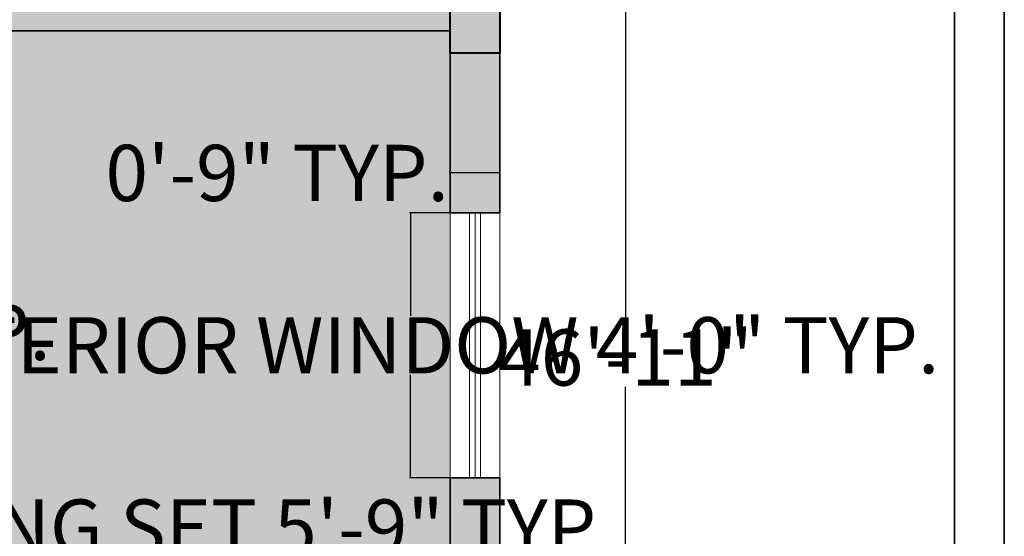
# Model space of a CAD drawing. Units: inches. Extents: x 1077 to 2505, y 1892 to 2728.
# Tile 16 of 26: x 1470 to 1648, y 2338 to 2431. Entities that reach past the tile are written whole.
import ezdxf

# ---------------------------------------------------------------- set-up
doc = ezdxf.new("R2010")
doc.units = ezdxf.units.IN
doc.linetypes.add('ACAD_ISO02W100', pattern=[15, 12, -3])
doc.layers.get('Defpoints').update_dxf_attribs({"color": 220, "linetype": 'ACAD_ISO02W100'})
for name, color, linetype, lineweight in [('A-ANNO-DIMS', 2, 'Continuous', 18), ('A-ANNO-TTLB', 7, 'Continuous', 35), ('A-COLS', 7, 'Continuous', 40), ('A-WALL-PATT', 7, 'Continuous', 9), ('WALL', 7, 'Continuous', 35), ('WINDOW', 160, 'Continuous', 13)]:
    doc.layers.add(name, color=color, linetype=linetype, lineweight=lineweight)
doc.layers.add('A-FLOR-PATT', color=254, linetype='Continuous', lineweight=9, true_color=0xd7ebd2)
doc.styles.get("Standard").update_dxf_attribs({"font": 'arial.ttf'})
doc.dimstyles.get("Standard").update_dxf_attribs({"dimtxt": 10.18, "dimasz": 0.18, "dimexe": 0.18, "dimexo": 0.0625, "dimgap": 0.09, "dimtad": 0, "dimtih": 1, "dimtoh": 1, "dimdec": 0, "dimzin": 0, "dimdsep": 46, "dimlunit": 3, "dimtxsty": 'Standard', "dimcen": 0.09, "dimadec": 0, "dimazin": 0, "dimtfac": 1, "dimtdec": 0, "dimtofl": 0, "dimtmove": 0, "dimatfit": 3, "dimfxl": 1, "dimtolj": 1, "dimtzin": 0, "dimarcsym": 0})

# ---------------------------------------------------------------- blocks, each defined once
blk = doc.blocks.new('C1')
h = blk.add_hatch(color=256)
h.dxf.hatch_style = 1
h.paths.add_polyline_path([(1668.56, 2445.41), (1677.56, 2445.41), (1677.56, 2457.41), (1668.56, 2457.41)])
for p, q in [((1668.56, 2457.41), (1677.56, 2457.41)), ((1668.56, 2445.41), (1668.56, 2457.41)), ((1677.56, 2457.41), (1677.56, 2445.41)), ((1677.56, 2445.41), (1668.56, 2445.41))]:
    blk.add_line(p, q)
blk = doc.blocks.new('*D14')
at = {"layer": 'A-ANNO-DIMS', "color": 0, "lineweight": -2, "transparency": 16777216}
for p, q in [((1555.59, 2651.66), (1579.43, 2651.66)), ((1579.25, 2651.48), (1579.25, 2375.3)), ((1579.25, 2088.54), (1579.25, 2364.72)), ((1555.59, 2088.36), (1579.43, 2088.36))]:
    blk.add_line(p, q, dxfattribs=at)
at = {"layer": 'A-ANNO-DIMS', "color": 0, "transparency": 16777216}
for points in [[(1579.22, 2651.48), (1579.28, 2651.48), (1579.25, 2651.66)], [(1579.22, 2088.54), (1579.28, 2088.54), (1579.25, 2088.36)]]:
    blk.add_solid(points, dxfattribs=at)
at = {"layer": 'Defpoints', "color": 0, "transparency": 16777216}
for p in [(1555.53, 2651.66), (1555.53, 2088.36), (1579.25, 2088.36)]:
    blk.add_point(p, dxfattribs=at)
at = {"layer": 'A-ANNO-DIMS', "color": 0, "transparency": 16777216, "insert": (1579.25, 2370.01), "char_height": 10.18, "attachment_point": 5}
blk.add_mtext('\\A1;46\'-11"', dxfattribs=at)
blk = doc.blocks.new('WINDOW-48-EXT')
for p, q in [((0, 48), (0, 0)), ((3.5, 48), (3.5, 0)), ((4.5, 48), (4.5, 0)), ((5.5, 48), (5.5, 0)), ((9, 0), (9, 48))]:
    blk.add_line(p, q)
blk = doc.blocks.new('SHEET-FRAME-RESIDENTIAL')
for points in [[(0, 830.04), (543.52, 830.04), (543.52, 0), (0, 0)], [(9, 821.04), (534.52, 821.04), (534.52, 9), (9, 9)]]:
    blk.add_lwpolyline(points, close=True)
blk = doc.blocks.new('*D36')
at = {"layer": 'A-ANNO-DIMS', "color": 0, "lineweight": -2, "transparency": 16777216}
for p, q in [((1365.09, 2349.48), (1365.09, 2339.05)), ((1433.87, 2349.48), (1433.87, 2339.05)), ((1365.27, 2339.23), (1433.69, 2339.23)), ((1433.87, 2339.23), (1434.05, 2339.23))]:
    blk.add_line(p, q, dxfattribs=at)
at = {"layer": 'A-ANNO-DIMS', "color": 0, "transparency": 16777216}
for points in [[(1365.27, 2339.26), (1365.27, 2339.2), (1365.09, 2339.23)], [(1433.69, 2339.26), (1433.69, 2339.2), (1433.87, 2339.23)]]:
    blk.add_solid(points, dxfattribs=at)
at = {"layer": 'Defpoints', "color": 0, "transparency": 16777216}
for p in [(1365.09, 2349.54), (1433.87, 2349.54), (1433.87, 2339.23)]:
    blk.add_point(p, dxfattribs=at)
at = {"layer": 'A-ANNO-DIMS', "color": 0, "transparency": 16777216, "insert": (1507.58, 2339.23), "char_height": 10.18, "attachment_point": 5}
blk.add_mtext('\\A1;DINING SET 5\'-9" TYP.', dxfattribs=at)
blk = doc.blocks.new('*D37')
at = {"layer": 'A-ANNO-DIMS', "color": 0, "lineweight": -2, "transparency": 16777216}
for p, q in [((1433.94, 2399.74), (1444.37, 2399.74)), ((1444.19, 2399.56), (1444.19, 2379.85)), ((1444.19, 2349.72), (1444.19, 2369.44)), ((1433.94, 2349.54), (1444.37, 2349.54))]:
    blk.add_line(p, q, dxfattribs=at)
at = {"layer": 'A-ANNO-DIMS', "color": 0, "transparency": 16777216}
for points in [[(1444.16, 2399.56), (1444.22, 2399.56), (1444.19, 2399.74)], [(1444.16, 2349.72), (1444.22, 2349.72), (1444.19, 2349.54)]]:
    blk.add_solid(points, dxfattribs=at)
at = {"layer": 'Defpoints', "color": 0, "transparency": 16777216}
for p in [(1433.87, 2399.74), (1444.19, 2399.74), (1433.87, 2349.54)]:
    blk.add_point(p, dxfattribs=at)
at = {"layer": 'A-ANNO-DIMS', "color": 0, "transparency": 16777216, "insert": (1444.19, 2374.64), "char_height": 10.18, "attachment_point": 5}
blk.add_mtext('\\A1;4\'-2" TYP.', dxfattribs=at)
blk = doc.blocks.new('*D58')
at = {"layer": 'A-ANNO-DIMS', "color": 0, "lineweight": -2, "transparency": 16777216}
for p, q in [((1547.47, 2396.22), (1540.15, 2396.22)), ((1540.33, 2396.04), (1540.33, 2377.58)), ((1540.33, 2348.4), (1540.33, 2366.87)), ((1547.47, 2348.22), (1540.15, 2348.22))]:
    blk.add_line(p, q, dxfattribs=at)
at = {"layer": 'A-ANNO-DIMS', "color": 0, "transparency": 16777216}
for points in [[(1540.3, 2396.04), (1540.36, 2396.04), (1540.33, 2396.22)], [(1540.3, 2348.4), (1540.36, 2348.4), (1540.33, 2348.22)]]:
    blk.add_solid(points, dxfattribs=at)
at = {"layer": 'Defpoints', "color": 0, "transparency": 16777216}
for p in [(1547.53, 2396.22), (1540.33, 2348.22), (1547.53, 2348.22)]:
    blk.add_point(p, dxfattribs=at)
at = {"layer": 'A-ANNO-DIMS', "color": 0, "transparency": 16777216, "insert": (1540.33, 2372.22), "char_height": 10.18, "attachment_point": 5}
blk.add_mtext('\\A1;EXTERIOR WINDOW 4\'-0" TYP.', dxfattribs=at)
blk = doc.blocks.new('*D59')
at = {"layer": 'A-ANNO-DIMS', "color": 0, "lineweight": -2, "transparency": 16777216}
for p, q in [((1547.53, 2403.42), (1547.35, 2403.42)), ((1547.53, 2396.29), (1547.53, 2403.6)), ((1556.35, 2403.42), (1547.71, 2403.42)), ((1556.53, 2396.29), (1556.53, 2403.6))]:
    blk.add_line(p, q, dxfattribs=at)
at = {"layer": 'A-ANNO-DIMS', "color": 0, "transparency": 16777216}
for points in [[(1547.71, 2403.45), (1547.71, 2403.39), (1547.53, 2403.42)], [(1556.35, 2403.45), (1556.35, 2403.39), (1556.53, 2403.42)]]:
    blk.add_solid(points, dxfattribs=at)
at = {"layer": 'Defpoints', "color": 0, "transparency": 16777216}
for p in [(1547.53, 2403.42), (1547.53, 2396.22), (1556.53, 2396.22)]:
    blk.add_point(p, dxfattribs=at)
at = {"layer": 'A-ANNO-DIMS', "color": 0, "transparency": 16777216, "insert": (1516.23, 2403.42), "char_height": 10.18, "attachment_point": 5}
blk.add_mtext('\\A1;0\'-9" TYP.', dxfattribs=at)

msp = doc.modelspace()

# ---------------------------------------------------------------- hatches: boundary and pattern name
at = {"layer": 'A-FLOR-PATT', "transparency": 33554559}
h = msp.add_hatch(color=256, dxfattribs=at)
h.dxf.hatch_style = 1
h.paths.add_polyline_path([(1395.53, 2577.16), (1374.83, 2577.16), (1350.83, 2577.19), (1350.83, 2577.16), (1329.53, 2577.16), (1329.53, 2480.16), (1329.53, 2469.16), (1325.53, 2469.16), (1325.53, 2515.13), (1307.53, 2515.13), (1307.53, 2577.16), (1269.31, 2577.16), (1221.31, 2577.15), (1221.31, 2577.16), (1187.53, 2577.16), (1187.53, 2433.16), (1289.53, 2433.16), (1289.53, 2429.16), (1263.53, 2429.16), (1187.53, 2429.16), (1187.53, 2395.02), (1187.53, 2395.02), (1187.53, 2371.02), (1187.53, 2371.02), (1187.53, 2307.16), (1259.53, 2307.16), (1259.53, 2399.16), (1263.53, 2399.16), (1263.53, 2307.16), (1289.53, 2307.16), (1289.53, 2306.23), (1325.53, 2306.23), (1325.53, 2307.16), (1329.53, 2307.16), (1329.53, 2306.23), (1365.53, 2306.23), (1365.53, 2307.16), (1432.53, 2307.16), (1432.53, 2088.16), (1547.53, 2088.16), (1547.53, 2140.08), (1511.53, 2140.08), (1511.53, 2267.16), (1475.53, 2267.16), (1475.53, 2303.16), (1468.53, 2303.16), (1468.53, 2307.16), (1547.53, 2307.16), (1547.53, 2348.22), (1547.53, 2396.22), (1547.53, 2429.16), (1435.53, 2429.16), (1435.53, 2433.16), (1476.35, 2433.16), (1476.35, 2451.18), (1547.53, 2451.18), (1547.53, 2577.16), (1499.53, 2577.16), (1499.53, 2586.16), (1547.53, 2586.16), (1547.53, 2642.16), (1518.18, 2642.16), (1518.18, 2642.05), (1494.15, 2642.05), (1494.15, 2642.16), (1469.53, 2642.16), (1469.53, 2577.16), (1399.53, 2577.16), (1399.53, 2429.16), (1325.53, 2429.16), (1325.53, 2433.16), (1329.53, 2433.16), (1395.53, 2433.16), (1395.53, 2480.16), (1359.53, 2480.16), (1359.53, 2484.16), (1395.53, 2484.16)])
h.paths.add_polyline_path([(1357.65, 2482.07), (1355.65, 2482.07), (1355.65, 2481.07, 0.414214), (1356.65, 2480.07), (1344.65, 2480.07), (1344.65, 2477.06), (1343.27, 2477.06), (1343.27, 2480.07), (1330.65, 2480.07, -0.414214), (1329.65, 2481.07), (1329.65, 2484.07), (1331.65, 2484.07), (1331.65, 2510.07, -0.446908)], flags=16)
h.paths.add_polyline_path([(1305.09, 2559.18), (1288.89, 2559.18), (1288.89, 2575.38), (1305.09, 2575.38)], flags=16)
h.paths.add_polyline_path([(1304.19, 2560.08), (1289.79, 2560.08), (1289.79, 2574.48), (1304.19, 2574.48)], flags=0)
h.paths.add_polyline_path([(1287.99, 2500.68, -0.414214), (1287.09, 2499.78), (1265.14, 2499.78), (1224.09, 2499.78, -0.414214), (1223.19, 2500.68), (1223.19, 2557.16), (1223.19, 2571.74), (1223.19, 2575.38), (1287.99, 2575.38), (1287.99, 2571.74), (1287.09, 2571.74, -0.414214), (1287.99, 2570.84)], flags=16)
h.paths.add_polyline_path([(1292.98, 2569.05, -1), (1300.92, 2569.05, -1)], flags=0)
h.paths.add_polyline_path([(1293.32, 2569.05, -1), (1300.58, 2569.05, -1)], flags=0)
h.paths.add_polyline_path([(1322.8, 2462.21), (1322.8, 2431.71), (1323.05, 2430.71), (1323.05, 2431.71), (1321.8, 2431.71), (1321.8, 2462.19, 0.404641), (1292.3, 2431.71), (1292.05, 2430.71, -0.414214), (1291.55, 2430.21), (1291.05, 2430.21), (1291.05, 2429.71, -0.414214), (1290.55, 2429.21), (1289.55, 2429.21), (1289.55, 2434.21), (1290.55, 2434.21, -0.414214), (1291.05, 2433.71), (1291.05, 2433.21), (1291.55, 2433.21, -0.414214), (1292.05, 2432.71), (1292.3, 2431.71, -0.414214)], flags=16)
h.paths.add_polyline_path([(1287.82, 2548.28, 0.292232), (1279.17, 2536.8, 0.052719), (1223.93, 2548.28), (1223.28, 2548.28), (1223.28, 2557.16), (1223.93, 2557.16), (1245.42, 2557.16, -0.117785), (1245.77, 2557.93, -0.059418), (1254.87, 2567.02, -0.379859), (1257.28, 2566.88, -0.02509), (1261.41, 2563.32, -0.025935), (1265.65, 2567.02, -0.379859), (1268.06, 2566.88, -0.061767), (1277.52, 2557.43, -0.069393), (1277.82, 2557.16), (1287.82, 2557.16)], flags=0)
h.paths.add_polyline_path([(1263.47, 2548.28), (1260.56, 2548.28, -0.015371), (1258.01, 2546.13, -0.429576), (1255.37, 2546.06, -0.016036), (1252.69, 2548.28), (1223.28, 2548.28), (1223.28, 2554.42), (1246.78, 2554.42, 0.055344), (1255.37, 2546.06, 0.331768), (1257.52, 2545.74, 0.027343), (1262, 2549.64, 0.00919)], flags=0)
h.paths.add_polyline_path([(1295.56, 2568.34), (1296.87, 2569.09), (1296.87, 2570.6, 0.399698), (1295.39, 2569.05, 0.119004)], flags=0)
h.paths.add_polyline_path([(1295.21, 2569.05, -1), (1298.68, 2569.05, -1)], flags=0)
h.paths.add_polyline_path([(1296.95, 2568.96), (1297.03, 2569), (1297.03, 2569.09), (1296.99, 2569.11), (1296.91, 2568.98)], flags=0)
h.paths.add_polyline_path([(1402.28, 2462.19, -0.414214), (1432.78, 2431.69), (1433.03, 2432.69), (1432.78, 2431.69, 0.404641), (1403.28, 2462.17), (1403.28, 2431.69), (1402.03, 2431.69), (1402.03, 2430.69, -0.414214), (1401.53, 2430.19), (1401.03, 2430.19), (1401.03, 2429.69, -0.414214), (1400.53, 2429.19), (1399.53, 2429.19), (1399.53, 2434.19), (1400.53, 2434.19, -0.414214), (1401.03, 2433.69), (1401.03, 2433.19), (1401.53, 2433.19, -0.414214), (1402.03, 2432.69)], flags=16)
h.paths.add_polyline_path([(1470.16, 2535.21, -0.414214), (1471.06, 2536.11), (1527.54, 2536.11), (1542.12, 2536.11), (1545.76, 2536.11), (1545.76, 2471.31), (1542.12, 2471.31), (1542.12, 2472.21, -0.414214), (1541.22, 2471.31), (1471.06, 2471.31, -0.414214), (1470.16, 2472.21), (1470.16, 2494.16)], flags=16)
h.paths.add_polyline_path([(1483.07, 2536.11, 0.253465), (1480.11, 2526.15, 0.2538), (1470.15, 2523.19)], flags=16)
h.paths.add_polyline_path([(1223.19, 2512.69, 0.253465), (1233.14, 2509.74, 0.2538), (1236.1, 2499.77)], flags=16)
h.paths.add_polyline_path([(1469.77, 2578.72), (1469.77, 2581.72), (1471.77, 2581.72), (1471.77, 2607.72, -0.01951), (1473.77, 2607.68), (1473.77, 2579.72), (1473.77, 2578.72, -0.414214), (1472.77, 2577.72), (1470.77, 2577.72, -0.414214)], flags=16)
h.paths.add_polyline_path([(1382.46, 2398.13), (1395.04, 2398.13), (1395.04, 2399.74), (1382.46, 2399.74)], flags=16)
h.paths.add_polyline_path([(1379.94, 2397.18), (1379.94, 2389.82), (1380.5, 2389.82), (1380.5, 2396.05, -0.41429), (1381.06, 2396.61), (1396.47, 2396.61, -0.414213), (1397.03, 2396.05), (1397.03, 2389.82), (1397.59, 2389.82), (1397.59, 2397.18)], flags=16)
h.paths.add_polyline_path([(1263.37, 2428.14), (1263.37, 2426.14, -0.414214), (1262.37, 2425.14), (1261.37, 2425.14), (1233.41, 2425.14, 0.400854), (1259.37, 2401.04), (1259.37, 2401.14), (1261.37, 2401.14, -0.446908), (1233.37, 2427.14), (1259.37, 2427.14), (1259.37, 2429.14), (1262.37, 2429.14, -0.414214)], flags=16)
h.paths.add_polyline_path([(1404.79, 2398.13), (1417.37, 2398.13), (1417.37, 2399.74), (1404.79, 2399.74)], flags=16)
h.paths.add_polyline_path([(1402.27, 2397.18), (1404.79, 2398.13), (1417.37, 2398.13), (1419.92, 2397.18)], flags=16)
h.paths.add_polyline_path([(1432.26, 2383.16), (1432.26, 2370.59), (1433.87, 2370.59), (1433.87, 2383.16)], flags=16)
h.paths.add_polyline_path([(1431.3, 2385.69), (1423.84, 2385.69), (1423.84, 2385.13), (1430.18, 2385.13, -0.41429), (1430.74, 2384.57), (1430.74, 2369.16, -0.414237), (1430.18, 2368.6), (1423.84, 2368.6), (1423.84, 2368.03), (1431.3, 2368.03)], flags=16)
h.paths.add_polyline_path([(1417.37, 2351.16), (1417.37, 2349.54), (1418.9, 2349.54, 0.414236), (1419.92, 2350.56), (1419.92, 2352.11)], flags=16)
h.paths.add_polyline_path([(1395.04, 2351.16), (1395.04, 2349.54), (1396.58, 2349.54, 0.414235), (1397.59, 2350.56), (1397.59, 2352.11)], flags=16)
h.paths.add_polyline_path([(1366.7, 2370.05), (1365.09, 2370.05), (1365.09, 2368.52, 0.414235), (1366.11, 2367.5), (1367.66, 2367.5)], flags=16)
h.paths.add_polyline_path([(1419.36, 2359.47), (1419.36, 2353.24, -0.41419), (1418.8, 2352.68), (1403.39, 2352.68, -0.414137), (1402.83, 2353.24), (1402.83, 2359.47), (1397.03, 2359.47), (1397.03, 2353.24, -0.414189), (1396.47, 2352.68), (1381.06, 2352.68, -0.414137), (1380.5, 2353.24), (1380.5, 2359.47)], flags=16)
h.paths.add_polyline_path([(1222.29, 2559.18), (1206.09, 2559.18), (1206.09, 2575.38), (1222.29, 2575.38)], flags=16)
h.paths.add_polyline_path([(1221.39, 2560.08), (1206.99, 2560.08), (1206.99, 2574.48), (1221.39, 2574.48)], flags=0)
h.paths.add_polyline_path([(1482, 2577.72), (1482, 2580.73), (1483.38, 2580.73), (1483.38, 2577.72), (1484.77, 2577.72), (1484.77, 2574.72), (1483.38, 2574.72), (1483.38, 2577.72)], flags=16)
h.paths.add_polyline_path([(1266.37, 2415.53), (1266.37, 2414.14), (1263.37, 2414.14), (1263.37, 2415.53), (1260.36, 2415.53), (1260.36, 2416.91), (1263.37, 2416.91), (1263.37, 2415.53)], flags=16)
h.paths.add_polyline_path([(1210.26, 2569.05, -1), (1218.19, 2569.05, -1)], flags=0)
h.paths.add_polyline_path([(1210.6, 2569.05, -1), (1217.85, 2569.05, -1)], flags=0)
h.paths.add_polyline_path([(1212.84, 2568.34), (1214.15, 2569.09), (1214.15, 2570.6, 0.399698), (1212.67, 2569.05, 0.119004)], flags=0)
h.paths.add_polyline_path([(1212.49, 2569.05, -1), (1215.96, 2569.05, -1)], flags=0)
h.paths.add_polyline_path([(1214.23, 2568.96), (1214.3, 2568.91), (1214.3, 2569)], flags=0)
h.paths.add_polyline_path([(1507.18, 2480.12, 0.052719), (1518.66, 2535.36), (1518.66, 2536.01), (1527.54, 2536.01), (1527.54, 2535.36), (1527.54, 2513.88, -0.117785), (1528.31, 2513.53, -0.059418), (1537.4, 2504.43, -0.379859), (1537.26, 2502.01, -0.02509), (1533.7, 2497.89, -0.025935), (1537.4, 2493.64, -0.379859), (1537.26, 2491.23, -0.061767), (1527.8, 2481.77, -0.069393), (1527.54, 2481.47), (1527.54, 2471.47), (1518.66, 2471.47, 0.292232)], flags=0)
h.paths.add_polyline_path([(1516.43, 2503.92, -0.016036), (1518.66, 2506.6), (1518.66, 2536.01), (1524.8, 2536.01), (1524.8, 2512.51, 0.055344), (1516.43, 2503.92, 0.331768), (1516.12, 2501.77, 0.027343), (1520.01, 2497.29, 0.00919), (1518.66, 2495.82), (1518.66, 2498.73, -0.015371), (1516.5, 2501.28, -0.429576)], flags=0)
h.paths.add_polyline_path([(1499.63, 2625.5, -0.171636), (1502.82, 2631.01), (1502.82, 2633.37), (1498.68, 2633.37, -0.414214), (1497.7, 2634.36), (1497.7, 2640.66, -0.414214), (1498.68, 2641.64), (1514.82, 2641.64, -0.414214), (1515.81, 2640.66), (1515.81, 2634.36, -0.414214), (1514.82, 2633.37), (1510.69, 2633.37), (1510.69, 2631.01, -0.171636), (1513.88, 2625.5, -0.258205), (1509.31, 2614.47), (1504.19, 2614.47, -0.258205)], flags=16)
h.paths.add_polyline_path([(1501.2, 2625.5, -0.171636), (1504.39, 2631.01), (1509.12, 2631.01, -0.171636), (1512.3, 2625.5, -0.210384), (1509.35, 2616.02), (1504.16, 2616.02, -0.210384)], flags=0)
h.paths.add_polyline_path([(1529.56, 2537.01), (1529.56, 2553.21), (1545.76, 2553.21), (1545.76, 2537.01)], flags=16)
h.paths.add_polyline_path([(1530.46, 2537.91), (1530.46, 2552.31), (1544.86, 2552.31), (1544.86, 2537.91)], flags=0)
h.paths.add_polyline_path([(1535.45, 2545.07, -1), (1543.39, 2545.07, -1)], flags=0)
h.paths.add_polyline_path([(1535.8, 2545.07, -1), (1543.05, 2545.07, -1)], flags=0)
h.paths.add_polyline_path([(1529.56, 2470.41), (1545.76, 2470.41), (1545.76, 2454.21), (1529.56, 2454.21)], flags=16)
h.paths.add_polyline_path([(1541.16, 2544.99), (1540.98, 2544.99, -0.544606), (1538.71, 2543.68), (1538.62, 2543.53, 0.547962)], flags=0)
h.paths.add_polyline_path([(1530.46, 2469.51), (1544.86, 2469.51), (1544.86, 2455.11), (1530.46, 2455.11)], flags=0)
h.paths.add_polyline_path([(1539.47, 2545.14), (1539.42, 2545.22), (1539.38, 2545.14)], flags=0)
h.paths.add_polyline_path([(1543.39, 2462.34, -1), (1535.45, 2462.34, -1)], flags=0)
h.paths.add_polyline_path([(1543.05, 2462.34, -1), (1535.8, 2462.34, -1)], flags=0)
h.paths.add_polyline_path([(1541.16, 2462.27), (1540.98, 2462.27, -0.544606), (1538.71, 2460.96), (1538.62, 2460.8, 0.547962)], flags=0)
h.paths.add_polyline_path([(1539.47, 2462.42), (1539.42, 2462.5), (1539.38, 2462.42)], flags=0)
h.paths.add_polyline_path([(1435.32, 2335.25, -0.414214), (1465.82, 2304.75), (1466.07, 2305.75), (1465.82, 2304.75, 0.404641), (1436.32, 2335.23), (1436.32, 2304.75), (1435.07, 2304.75), (1435.07, 2303.75, -0.414214), (1434.57, 2303.25), (1434.07, 2303.25), (1434.07, 2302.75, -0.414214), (1433.57, 2302.25), (1432.57, 2302.25), (1432.57, 2307.25), (1433.57, 2307.25, -0.414214), (1434.07, 2306.75), (1434.07, 2306.25), (1434.57, 2306.25, -0.414214), (1435.07, 2305.75)], flags=16)
h.paths.add_polyline_path([(1532.13, 2635.71), (1535.43, 2635.71), (1535.43, 2635.89), (1532.13, 2635.89)], flags=16)
edge = h.paths.add_edge_path(flags=16)
edge.add_arc((1535.98, 2632.67), 0.183, 270, 360)
edge.add_line((1536.17, 2632.67), (1536.17, 2639.82))
edge.add_line((1536.17, 2639.82), (1538.29, 2639.82))
edge.add_line((1538.29, 2639.82), (1538.29, 2641.82))
edge.add_line((1538.29, 2641.82), (1533.25, 2641.82))
edge.add_line((1533.25, 2641.82), (1533.25, 2639.82))
edge.add_line((1533.25, 2639.82), (1534.87, 2639.82))
edge.add_line((1534.87, 2639.82), (1534.87, 2639))
edge.add_line((1534.87, 2639), (1533.7, 2639))
edge.add_line((1533.7, 2639), (1533.7, 2639.82))
edge.add_line((1533.7, 2639.82), (1533.25, 2639.82))
edge.add_line((1533.25, 2639.82), (1533.25, 2641.82))
edge.add_line((1533.25, 2641.82), (1538.29, 2641.82))
edge.add_line((1538.29, 2641.82), (1538.29, 2641.34))
edge.add_line((1538.29, 2641.34), (1540.64, 2641.58))
edge.add_line((1540.64, 2641.58), (1540.64, 2641.82))
edge.add_line((1540.64, 2641.82), (1541.5, 2641.82))
edge.add_line((1541.5, 2641.82), (1541.5, 2641.25))
edge.add_line((1541.5, 2641.25), (1541.31, 2639.79))
edge.add_ellipse((1541.09, 2638.95), major_axis=(-1.08, 0), ratio=0.790849, start_angle=180, end_angle=255.2976, ccw=False)
edge.add_line((1542.17, 2638.95), (1542.17, 2638.38))
edge.add_ellipse((1541.09, 2638.38), major_axis=(-1.08, 0), ratio=0.790849, start_angle=0, end_angle=180, ccw=False)
edge.add_line((1540, 2638.38), (1540.01, 2638.87))
edge.add_ellipse((1541.09, 2638.95), major_axis=(-1.08, 0), ratio=0.790849, start_angle=284.7024, end_angle=364.0401, ccw=False)
edge.add_line((1540.78, 2639.75), (1540.78, 2641.25))
edge.add_line((1540.78, 2641.25), (1540.64, 2641.25))
edge.add_line((1540.64, 2641.25), (1538.29, 2641.01))
edge.add_line((1538.29, 2641.01), (1538.29, 2639.82))
edge.add_line((1538.29, 2639.82), (1536.17, 2639.82))
edge.add_line((1536.17, 2639.82), (1536.17, 2632.48))
edge.add_line((1536.17, 2632.48), (1535.98, 2632.48))
h.paths.add_polyline_path([(1496.32, 2250.34, -0.292371), (1498.9, 2247.83, -0.085148), (1501.21, 2208.85, -0.01331), (1500.27, 2098.5, -0.379287), (1497.22, 2095.28, -0.0502), (1441.54, 2095.28, -0.379287), (1438.5, 2098.5, -0.01331), (1437.56, 2208.85, -0.086132), (1439.96, 2248.26, -0.295116), (1442.59, 2250.78, -0.114238)], flags=16)
h.paths.add_polyline_path([(1495.16, 2205.84, -0.355389), (1496.7, 2202.1), (1492.94, 2189.65, -0.398275), (1489.12, 2187.47, 0.113332), (1449.64, 2187.47, -0.398275), (1445.82, 2189.65), (1442.06, 2202.1, -0.355394), (1443.6, 2205.84, -0.265725)], flags=0)
h.paths.add_polyline_path([(1440.37, 2195.72), (1445.94, 2181.67), (1445.94, 2160.63), (1440.84, 2157.26)], flags=0)
h.paths.add_polyline_path([(1498.46, 2195.72), (1497.99, 2157.26), (1492.88, 2160.63), (1492.88, 2181.67)], flags=0)
h.paths.add_polyline_path([(1445.94, 2158.37), (1445.94, 2137.12), (1441.12, 2122.56), (1440.87, 2155.03)], flags=0)
h.paths.add_polyline_path([(1492.88, 2158.37), (1497.96, 2155.03), (1497.71, 2122.56), (1492.88, 2137.12)], flags=0)
h.paths.add_polyline_path([(1489.88, 2130.4), (1494.39, 2107.67, -0.090102), (1444.44, 2107.65), (1448.95, 2130.39, 0.036636)], flags=0)
h.paths.add_polyline_path([(1447.54, 2159.34), (1497.44, 2159.34), (1497.44, 2177.89), (1447.54, 2177.89)], flags=8)
h.paths.add_polyline_path([(1196.44, 2354.84), (1246.65, 2354.84), (1246.65, 2388.43), (1196.44, 2388.43)], flags=24)
h.paths.add_polyline_path([(1296.09, 2360.25), (1353.81, 2360.25), (1353.81, 2393.84), (1296.09, 2393.84)], flags=24)
h.paths.add_polyline_path([(1400.72, 2471.85), (1470.63, 2471.85), (1470.63, 2505.44), (1400.72, 2505.44)], flags=24)
h.paths.add_polyline_path([(1324.78, 2448.48), (1394.95, 2448.48), (1394.95, 2467.02), (1324.78, 2467.02)], flags=24)
h.paths.add_polyline_path([(1335.08, 2531.43), (1389.67, 2531.43), (1389.67, 2565.02), (1335.08, 2565.02)], flags=24)
h.paths.add_polyline_path([(1225.76, 2460), (1295.67, 2460), (1295.67, 2493.58), (1225.76, 2493.58)], flags=24)
h = msp.add_hatch(color=256, dxfattribs=at)
h.dxf.hatch_style = 1
h.paths.add_polyline_path([(1547.53, 2348.22), (1547.53, 2396.22), (1547.53, 2425.11), (1547.53, 2425.11), (1547.53, 2429.16), (1435.53, 2429.16), (1434.03, 2429.21), (1434.03, 2430.19), (1433.03, 2430.19), (1432.78, 2431.69, 0.404641), (1403.28, 2462.17), (1403.28, 2431.69), (1402.03, 2431.69), (1402.03, 2430.19), (1401.03, 2430.19), (1401.03, 2429.19), (1399.53, 2429.19), (1399.53, 2429.19), (1399.53, 2429.16), (1334.67, 2429.16), (1334.67, 2423.95), (1325.67, 2423.95), (1325.67, 2429.16), (1325.53, 2429.16), (1324.05, 2429.24), (1324.05, 2430.21), (1323.05, 2430.21), (1323.05, 2431.71), (1321.8, 2431.71), (1321.8, 2462.19, 0.416544), (1292.05, 2430.73, -0.423614), (1291.55, 2430.21), (1291.05, 2430.21), (1291.05, 2429.21), (1289.55, 2429.21), (1289.53, 2429.21), (1289.53, 2429.16), (1263.37, 2429.16), (1263.37, 2415.53), (1266.37, 2415.53), (1266.37, 2414.14), (1263.37, 2414.14), (1263.37, 2399.16), (1263.53, 2399.16), (1263.53, 2307.16), (1289.53, 2307.16), (1289.53, 2306.23), (1323.26, 2306.23), (1323.26, 2307.21), (1332.26, 2307.21), (1365.53, 2306.23), (1365.53, 2307.16), (1432.53, 2307.16), (1432.57, 2307.16), (1432.57, 2307.25), (1434.07, 2307.25), (1434.07, 2306.25), (1435.32, 2306.25), (1435.32, 2335.25, -0.407346), (1466.07, 2305.73, -0.423614), (1466.57, 2306.25), (1467.07, 2306.25), (1467.07, 2307.25), (1468.57, 2307.25), (1547.53, 2307.16), (1547.53, 2307.2)])
h.paths.add_polyline_path([(1430.74, 2369.16), (1430.74, 2384.57, 0.41429), (1430.18, 2385.13), (1423.84, 2385.13), (1423.84, 2368.6), (1430.18, 2368.6, 0.414237)], flags=16)
h.paths.add_polyline_path([(1432.26, 2383.16), (1432.26, 2370.59), (1433.87, 2370.59), (1433.87, 2383.16)], flags=16)
h.paths.add_polyline_path([(1431.3, 2368.03), (1431.3, 2385.69), (1432.26, 2383.16), (1432.26, 2370.59)], flags=16)
h.paths.add_polyline_path([(1417.37, 2351.16), (1417.37, 2349.54), (1418.9, 2349.54, 0.414236), (1419.92, 2350.56), (1419.92, 2352.11)], flags=16)
h.paths.add_polyline_path([(1403.39, 2352.68), (1418.78, 2352.68, 0.42427), (1419.36, 2353.24), (1419.36, 2359.47), (1402.83, 2359.47), (1402.83, 2353.24, 0.414137)], flags=16)
h.paths.add_polyline_path([(1366.7, 2370.05), (1365.09, 2370.05), (1365.09, 2368.52, 0.414235), (1366.11, 2367.5), (1367.66, 2367.5)], flags=16)
h.paths.add_polyline_path([(1382.46, 2398.13), (1395.04, 2398.13), (1395.04, 2399.74), (1382.46, 2399.74)], flags=16)
h.paths.add_polyline_path([(1396.47, 2396.61), (1381.06, 2396.61, 0.41429), (1380.5, 2396.05), (1380.5, 2389.82), (1397.03, 2389.82), (1397.03, 2396.05, 0.414213)], flags=16)
h.paths.add_polyline_path([(1402.27, 2397.18), (1402.83, 2396.05, -0.414213), (1403.39, 2396.61)], flags=16)
h.paths.add_polyline_path([(1418.8, 2396.61), (1419.36, 2396.61), (1419.36, 2396.05, 0.414237)], flags=16)
h.paths.add_polyline_path([(1404.79, 2398.13), (1417.37, 2398.13), (1417.37, 2399.74), (1404.79, 2399.74)], flags=16)
h.paths.add_polyline_path([(1381.06, 2352.68, -0.414213), (1380.5, 2353.24), (1380.27, 2352.11)], flags=16)
h.paths.add_polyline_path([(1396.58, 2349.54), (1396.58, 2349.54), (1395.04, 2349.54), (1395.04, 2349.54), (1382.46, 2349.54), (1382.46, 2351.16), (1395.04, 2351.16), (1397.59, 2352.11), (1397.59, 2350.56, -0.414235)], flags=16)
h.paths.add_polyline_path([(1379.94, 2397.18), (1382.46, 2398.13), (1395.04, 2398.13), (1397.59, 2397.18)], flags=16)
h.paths.add_polyline_path([(1368.78, 2384.59, 0.414213), (1368.22, 2384.03), (1367.66, 2367.5), (1367.66, 2385.15)], flags=16)
h.paths.add_polyline_path([(1547.53, 2574.38), (1547.51, 2574.38), (1547.51, 2577.16), (1499.53, 2577.16), (1484.77, 2577.44), (1484.77, 2574.72), (1483.38, 2574.72), (1483.38, 2577.72), (1482, 2577.72), (1469.53, 2577.72), (1469.53, 2577.16), (1401.95, 2577.16), (1401.95, 2574.12), (1399.53, 2574.12), (1399.53, 2434.19), (1401.03, 2434.19), (1401.03, 2433.19), (1402.28, 2433.19), (1402.28, 2462.19, -0.407346), (1433.03, 2432.67, -0.423614), (1433.53, 2433.19), (1434.03, 2433.19), (1434.03, 2434.19), (1435.53, 2434.19), (1476.35, 2433.81), (1476.35, 2451.18), (1547.53, 2451.18)])
h.paths.add_polyline_path([(1470.16, 2535.21, -0.414214), (1471.06, 2536.11), (1527.54, 2536.11), (1542.12, 2536.11), (1545.76, 2536.11), (1545.76, 2471.31), (1542.12, 2471.31), (1542.12, 2472.21, -0.414214), (1541.22, 2471.31), (1471.06, 2471.31, -0.414214), (1470.16, 2472.21), (1470.16, 2494.16)], flags=16)
h.paths.add_polyline_path([(1483.07, 2536.11, 0.253465), (1480.11, 2526.15, 0.2538), (1470.15, 2523.19)], flags=16)
h.paths.add_polyline_path([(1525.55, 2481.52, -0.000893), (1524.8, 2482.24), (1524.8, 2471.47), (1527.54, 2471.47), (1527.54, 2472.12), (1527.54, 2481.47, -0.388819)], flags=0)
h.paths.add_polyline_path([(1518.66, 2536.01), (1527.54, 2536.01), (1527.54, 2535.36), (1527.54, 2513.88, -0.117785), (1528.31, 2513.53, -0.059418), (1537.4, 2504.43, -0.379859), (1537.26, 2502.01, -0.02509), (1533.7, 2497.89, 0.033431), (1528.3, 2502.74, 0.308459), (1526.25, 2502.88, 0.047827), (1518.66, 2495.82), (1518.66, 2498.73, -0.015371), (1516.5, 2501.28, -0.429576), (1516.43, 2503.92, -0.016036), (1518.66, 2506.6)], flags=0)
h.paths.add_polyline_path([(1529.56, 2537.01), (1529.56, 2553.21), (1545.76, 2553.21), (1545.76, 2537.01)], flags=16)
h.paths.add_polyline_path([(1530.46, 2537.91), (1530.46, 2552.31), (1544.86, 2552.31), (1544.86, 2537.91)], flags=0)
h.paths.add_polyline_path([(1535.8, 2545.07, -1), (1543.05, 2545.07, -1)], flags=0)
h.paths.add_polyline_path([(1541.16, 2544.99), (1540.98, 2544.99, -0.544606), (1538.71, 2543.68), (1538.62, 2543.53, 0.547962)], flags=0)
h.paths.add_polyline_path([(1539.47, 2545.14), (1539.42, 2545.22), (1539.38, 2545.14)], flags=0)
h.paths.add_polyline_path([(1529.56, 2470.41), (1545.76, 2470.41), (1545.76, 2454.21), (1529.56, 2454.21)], flags=16)
h.paths.add_polyline_path([(1530.46, 2469.51), (1544.86, 2469.51), (1544.86, 2455.11), (1530.46, 2455.11)], flags=0)
h.paths.add_polyline_path([(1535.8, 2462.34, -1), (1543.05, 2462.34, -1)], flags=0)
h.paths.add_polyline_path([(1541.16, 2462.27), (1540.98, 2462.27, -0.544606), (1538.71, 2460.96), (1538.62, 2460.8, 0.547962)], flags=0)
h.paths.add_polyline_path([(1539.47, 2462.42), (1539.42, 2462.5), (1539.38, 2462.42)], flags=0)
h.paths.add_polyline_path([(1395.53, 2574.12), (1392.95, 2574.12), (1392.95, 2577.16), (1374.83, 2577.16), (1350.83, 2577.19), (1350.83, 2577.16), (1332.07, 2577.16), (1332.07, 2574), (1329.53, 2574), (1329.53, 2484.07), (1331.65, 2484.07), (1331.65, 2510.07, -0.423677), (1357.76, 2484.07), (1359.53, 2484.07), (1359.53, 2484.16), (1395.53, 2484.16)], flags=17)
h.paths.add_polyline_path([(1395.53, 2480.16), (1359.06, 2480.16, 0.437533), (1359.53, 2481.55), (1359.53, 2484.16), (1395.53, 2484.16), (1395.53, 2574.12), (1392.95, 2574.12), (1392.95, 2577.16), (1374.83, 2577.16), (1350.83, 2577.19), (1350.83, 2577.16), (1332.07, 2577.16), (1332.07, 2574), (1329.53, 2574), (1329.53, 2484.07), (1329.65, 2484.07), (1329.65, 2481.07), (1329.53, 2480.16), (1329.53, 2469.16), (1325.53, 2469.16), (1325.53, 2515.13), (1307.53, 2515.13), (1307.53, 2577.16), (1269.31, 2577.16), (1221.31, 2577.15), (1221.31, 2577.16), (1187.61, 2577.16), (1187.61, 2574.03), (1187.53, 2433.16), (1289.55, 2433.16), (1289.55, 2434.21), (1291.05, 2434.21), (1291.05, 2433.21), (1292.05, 2433.21), (1292.3, 2431.71, -0.414214), (1322.8, 2462.21), (1323.05, 2432.71, -0.414214), (1323.55, 2433.21), (1324.05, 2433.21), (1324.05, 2434.21), (1325.67, 2434.21), (1325.67, 2435.95), (1334.67, 2435.95), (1334.67, 2433.16), (1395.53, 2433.16)])
h.paths.add_polyline_path([(1344.65, 2480.07), (1344.65, 2477.06), (1343.27, 2477.06), (1343.27, 2480.07), (1332.65, 2480.07, 0.414214), (1333.65, 2481.07), (1333.65, 2482.07), (1331.65, 2482.07), (1331.65, 2484.07), (1331.65, 2510.07, -0.446908), (1357.65, 2482.07), (1355.65, 2482.07), (1355.65, 2481.07, 0.414214), (1356.65, 2480.07)], flags=16)
h.paths.add_polyline_path([(1287.99, 2500.68, -0.414214), (1287.09, 2499.78), (1265.14, 2499.78), (1224.09, 2499.78, -0.414214), (1223.19, 2500.68), (1223.19, 2557.16), (1223.19, 2571.74), (1223.19, 2575.38), (1287.99, 2575.38), (1287.99, 2571.74), (1287.09, 2571.74, -0.414214), (1287.99, 2570.84)], flags=16)
h.paths.add_polyline_path([(1277.77, 2555.17, -0.000893), (1277.05, 2554.42), (1287.82, 2554.42), (1287.82, 2557.16), (1287.17, 2557.16), (1277.82, 2557.16, -0.388819)], flags=0)
h.paths.add_polyline_path([(1223.28, 2548.28), (1223.28, 2557.16), (1223.93, 2557.16), (1245.42, 2557.16, -0.117785), (1245.77, 2557.93, -0.059418), (1254.87, 2567.02, -0.379859), (1257.28, 2566.88, -0.02509), (1261.41, 2563.32, 0.033431), (1256.55, 2557.93, 0.308459), (1256.41, 2555.88, 0.047827), (1263.47, 2548.28), (1260.56, 2548.28, -0.015371), (1258.01, 2546.13, -0.429576), (1255.37, 2546.06, -0.016036), (1252.69, 2548.28)], flags=0)
h.paths.add_polyline_path([(1305.09, 2559.18), (1288.89, 2559.18), (1288.89, 2575.38), (1305.09, 2575.38)], flags=16)
h.paths.add_polyline_path([(1304.19, 2560.08), (1289.79, 2560.08), (1289.79, 2574.48), (1304.19, 2574.48)], flags=0)
h.paths.add_polyline_path([(1300.58, 2569.05, -1), (1293.32, 2569.05, -1)], flags=0)
h.paths.add_polyline_path([(1223.19, 2512.69, 0.253465), (1233.14, 2509.74, 0.2538), (1236.1, 2499.77)], flags=16)
h.paths.add_polyline_path([(1295.56, 2568.34), (1296.87, 2569.09), (1296.87, 2570.6, 0.399698), (1295.39, 2569.05, 0.119004)], flags=0)
h.paths.add_polyline_path([(1295.21, 2569.05, -1), (1298.68, 2569.05, -1)], flags=0)
h.paths.add_polyline_path([(1296.95, 2568.96), (1297.03, 2569), (1297.03, 2569.09), (1296.99, 2569.11), (1296.91, 2568.98)], flags=0)
h.paths.add_polyline_path([(1222.29, 2559.18), (1206.09, 2559.18), (1206.09, 2575.38), (1222.29, 2575.38)], flags=16)
h.paths.add_polyline_path([(1221.39, 2560.08), (1206.99, 2560.08), (1206.99, 2574.48), (1221.39, 2574.48)], flags=0)
h.paths.add_polyline_path([(1217.85, 2569.05, -1), (1210.6, 2569.05, -1)], flags=0)
h.paths.add_polyline_path([(1212.84, 2568.34), (1214.15, 2569.09), (1214.15, 2570.6, 0.399698), (1212.67, 2569.05, 0.119004)], flags=0)
h.paths.add_polyline_path([(1212.49, 2569.05, -1), (1215.96, 2569.05, -1)], flags=0)
h.paths.add_polyline_path([(1214.23, 2568.96), (1214.3, 2569), (1214.3, 2569.09), (1214.26, 2569.11), (1214.19, 2568.98)], flags=0)
h.paths.add_polyline_path([(1259.53, 2399.14), (1259.37, 2399.14), (1259.37, 2401.04, -0.423677), (1233.37, 2427.14), (1259.37, 2427.14), (1259.37, 2429.16), (1187.53, 2429.16), (1187.53, 2395.02), (1187.53, 2395.02), (1187.53, 2371.02), (1187.53, 2371.02), (1187.53, 2311.49), (1187.55, 2311.49), (1187.55, 2307.16), (1259.53, 2307.16)])
h.paths.add_polyline_path([(1323.26, 2295.21), (1323.26, 2304.23), (1289.53, 2304.23), (1289.53, 2303.16), (1187.55, 2303.16), (1187.55, 2299.49), (1178.53, 2299.49), (1178.53, 2267.66), (1178.53, 2219.66), (1182.03, 2219.66), (1182.03, 2267.67), (1184.03, 2267.67), (1184.03, 2219.66), (1187.53, 2219.66), (1187.53, 2153.16), (1228.13, 2153.16), (1276.13, 2153.16), (1276.13, 2153.16), (1324.54, 2153.16), (1324.54, 2154.67), (1325.54, 2154.67), (1325.54, 2155.92), (1296.54, 2155.92, -0.407346), (1326.06, 2186.67, -0.423614), (1325.54, 2187.17), (1325.54, 2187.67), (1324.54, 2187.67), (1324.54, 2189.17), (1325.43, 2295.21)])
h.paths.add_polyline_path([(1432.53, 2307.16), (1365.53, 2307.16), (1365.53, 2306.23), (1365.53, 2303.16), (1428.53, 2303.16), (1428.53, 2221.2), (1428.57, 2221.2), (1428.57, 2197.2), (1428.53, 2197.16), (1428.53, 2303.01), (1404.46, 2303.01), (1404.46, 2221.2), (1329.53, 2221.2), (1329.53, 2307.16), (1325.53, 2307.16), (1325.53, 2295.21), (1325.43, 2295.21), (1324.54, 2189.17), (1324.54, 2187.67), (1326.04, 2187.67, 1.016365), (1326.06, 2186.67, 0.407348), (1296.54, 2155.92), (1325.54, 2155.92), (1325.54, 2154.67), (1324.54, 2154.67), (1324.54, 2153.16), (1329.53, 2153.16), (1329.53, 2144.16), (1432.53, 2144.16)])
h.paths.add_polyline_path([(1361.95, 2194.26), (1361.95, 2193.16), (1329.53, 2193.16), (1329.53, 2189.16), (1329.54, 2188.17), (1329.54, 2189.16), (1329.53, 2189.16), (1329.53, 2193.16), (1361.95, 2193.16), (1361.95, 2196.26), (1409.95, 2196.26), (1409.95, 2194.26)], flags=16)
h.paths.add_polyline_path([(1377.02, 2200.5), (1345.91, 2200.5), (1345.91, 2218.4), (1347.87, 2218.4), (1347.87, 2219.18), (1374.75, 2219.18), (1374.75, 2218.4), (1377.02, 2218.4)], flags=16)
h.paths.add_polyline_path([(1367.07, 2210.7, -1), (1373.34, 2210.7, -1)], flags=0)
h.paths.add_polyline_path([(1349.92, 2210.7, -1), (1356.98, 2210.7, -1)], flags=0)
h.paths.add_polyline_path([(1405.95, 2256.57), (1405.95, 2277.6), (1427.86, 2277.6), (1427.86, 2256.57)], flags=16)
h.paths.add_polyline_path([(1412.92, 2258.68, -0.414201), (1410.93, 2260.67), (1410.93, 2273.62, -0.414239), (1412.92, 2275.61), (1423.88, 2275.61, -0.414227), (1425.87, 2273.62), (1425.87, 2260.67, -0.414214), (1423.88, 2258.68)], flags=0)
h.paths.add_polyline_path([(1407.61, 2263.66, -1), (1409.18, 2263.66, -1)], flags=0)
h.paths.add_polyline_path([(1407.61, 2267.14, -1), (1409.18, 2267.14, -1)], flags=0)
h.paths.add_polyline_path([(1416.91, 2267.15, -1), (1419.89, 2267.15, -1)], flags=0)
h.paths.add_polyline_path([(1407.61, 2270.63, -1), (1409.18, 2270.63, -1)], flags=0)
h.paths.add_polyline_path([(1475.53, 2303.16), (1468.57, 2303.16), (1468.57, 2302.25), (1467.07, 2302.25), (1467.07, 2303.25), (1466.07, 2303.25), (1465.82, 2304.75, 0.404641), (1436.32, 2335.23), (1436.32, 2304.75), (1435.07, 2304.75), (1435.07, 2303.25), (1434.07, 2303.25), (1434.07, 2302.25), (1432.53, 2302.25), (1432.53, 2144.16), (1432.53, 2088.16), (1547.52, 2088.16), (1547.52, 2100.19), (1547.52, 2140.08), (1511.53, 2140.08), (1511.53, 2267.16), (1475.53, 2267.16)])
h.paths.add_polyline_path([(1438.35, 2102.86, 0.033498), (1438.37, 2102.21, -0.000079)], flags=16)
h.paths.add_polyline_path([(1496.32, 2250.34, -0.292371), (1498.9, 2247.83, -0.085148), (1501.21, 2208.85, -0.012784), (1500.42, 2102.86, -0.033498), (1500.39, 2102.21, 0.012863), (1501.21, 2208.85, 0.077283), (1499.67, 2244.3, 0.265882), (1497.48, 2246.8, 0.14401), (1441.46, 2247.36, 0.270646), (1439.21, 2244.85, -0.007564), (1439.96, 2248.26, -0.295116), (1442.59, 2250.78, -0.114238)], flags=16)
h.paths.add_polyline_path([(1495.16, 2205.84, -0.355389), (1496.7, 2202.1), (1492.94, 2189.65, -0.398275), (1489.12, 2187.47, 0.113332), (1449.64, 2187.47, -0.398275), (1445.82, 2189.65), (1442.06, 2202.1, -0.355394), (1443.6, 2205.84, -0.265725)], flags=16)
h.paths.add_polyline_path([(1440.37, 2195.72), (1445.94, 2181.67), (1445.94, 2160.63), (1440.84, 2157.26)], flags=16)
h.paths.add_polyline_path([(1498.46, 2195.72), (1497.99, 2157.26), (1492.88, 2160.63), (1492.88, 2181.67)], flags=16)
h.paths.add_polyline_path([(1445.94, 2158.37), (1445.94, 2137.12), (1441.12, 2122.56), (1440.87, 2155.03)], flags=16)
h.paths.add_polyline_path([(1492.88, 2158.37), (1497.96, 2155.03), (1497.71, 2122.56), (1492.88, 2137.12)], flags=16)
h.paths.add_polyline_path([(1489.88, 2130.4), (1494.39, 2107.67, -0.090102), (1444.44, 2107.65), (1448.95, 2130.39, 0.036636)], flags=16)
h.paths.add_polyline_path([(1296.09, 2360.25), (1353.81, 2360.25), (1353.81, 2393.84), (1296.09, 2393.84)], flags=24)
h.paths.add_polyline_path([(1400.72, 2471.85), (1470.63, 2471.85), (1470.63, 2505.44), (1400.72, 2505.44)], flags=24)
h.paths.add_polyline_path([(1335.08, 2531.43), (1389.67, 2531.43), (1389.67, 2565.02), (1335.08, 2565.02)], flags=24)
h.paths.add_polyline_path([(1324.78, 2448.48), (1394.95, 2448.48), (1394.95, 2467.02), (1324.78, 2467.02)], flags=24)
h.paths.add_polyline_path([(1225.76, 2460), (1295.67, 2460), (1295.67, 2493.58), (1225.76, 2493.58)], flags=24)
h.paths.add_polyline_path([(1196.44, 2354.84), (1246.65, 2354.84), (1246.65, 2388.43), (1196.44, 2388.43)], flags=24)
h.paths.add_polyline_path([(1447.54, 2159.34), (1497.44, 2159.34), (1497.44, 2177.89), (1447.54, 2177.89)], flags=24)
at = {"layer": 'A-WALL-PATT', "transparency": 33554585}
h = msp.add_hatch(color=256, dxfattribs=at)
h.dxf.hatch_style = 1
h.paths.add_polyline_path([(1187.53, 2424), (1178.53, 2424), (1178.53, 2395.02), (1187.53, 2395.02)])
h.paths.add_polyline_path([(1187.53, 2371.02), (1178.53, 2371.02), (1178.53, 2311.49), (1187.53, 2311.49)])
h.paths.add_polyline_path([(1228.13, 2153.16), (1187.53, 2153.16), (1187.53, 2219.66), (1178.53, 2219.66), (1178.53, 2100.18), (1187.53, 2100.18), (1187.53, 2144.16), (1228.13, 2144.16)])
h.paths.add_polyline_path([(1432.53, 2097.16), (1187.53, 2097.16), (1187.53, 2100.18), (1178.53, 2100.18), (1178.53, 2088.16), (1432.53, 2088.16)])
h.paths.add_polyline_path([(1556.53, 2348.22), (1547.53, 2348.22), (1547.53, 2348.22), (1547.53, 2307.16), (1468.53, 2307.16), (1468.53, 2303.16), (1547.53, 2303.16), (1547.53, 2088.16), (1556.53, 2088.16)])
h.paths.add_polyline_path([(1556.53, 2425.11), (1547.53, 2425.11), (1547.53, 2396.22), (1556.53, 2396.22)])
h.paths.add_polyline_path([(1547.53, 2433.16), (1435.53, 2433.16), (1435.53, 2429.16), (1547.53, 2429.16)])
h.paths.add_polyline_path([(1556.53, 2574.38), (1547.53, 2574.38), (1547.53, 2451.18), (1547.55, 2451.18), (1547.55, 2437.11), (1556.53, 2437.11)])
h.paths.add_polyline_path([(1556.53, 2639.11), (1547.53, 2639.11), (1547.53, 2586.38), (1556.53, 2586.38)])
h.paths.add_polyline_path([(1556.53, 2639.11), (1547.53, 2639.11), (1547.53, 2642.16), (1518.18, 2642.16), (1518.18, 2642.05), (1494.18, 2642.05), (1494.18, 2651.05), (1518.15, 2651.05), (1518.15, 2651.16), (1556.53, 2651.16)])
h.paths.add_polyline_path([(1494.15, 2651.16), (1469.6, 2651.16), (1469.6, 2642.16), (1494.15, 2642.16)])
h.paths.add_polyline_path([(1221.31, 2577.16), (1187.61, 2577.16), (1187.61, 2574.03), (1178.61, 2574.03), (1178.61, 2586.16), (1221.31, 2586.16)])
h.paths.add_polyline_path([(1323.07, 2586.16), (1269.31, 2586.16), (1269.31, 2577.16), (1323.07, 2577.16)])
h.paths.add_polyline_path([(1374.84, 2586.19), (1374.84, 2577.19), (1350.84, 2577.19), (1350.83, 2577.19), (1350.83, 2577.16), (1332.07, 2577.16), (1332.07, 2574), (1323.07, 2574), (1323.07, 2586.16), (1350.83, 2586.16), (1350.84, 2586.16), (1350.84, 2586.19)])
h.paths.add_polyline_path([(1392.95, 2586.16), (1374.84, 2586.16), (1374.84, 2577.16), (1392.95, 2577.16)], flags=17)
h.paths.add_polyline_path([(1469.53, 2642.16), (1469.6, 2651.16), (1460.53, 2651.16), (1460.53, 2586.16), (1392.95, 2586.16), (1392.95, 2577.16), (1395.53, 2577.16), (1395.53, 2484.16), (1359.53, 2484.16), (1359.53, 2480.16), (1395.53, 2480.16), (1395.53, 2433.16), (1329.53, 2433.16), (1325.53, 2433.16), (1325.53, 2429.16), (1399.53, 2429.16), (1399.53, 2577.16), (1469.53, 2577.16)])
h.paths.add_polyline_path([(1187.53, 2574.03), (1178.53, 2574.03), (1178.53, 2436), (1187.53, 2436)])

# ---------------------------------------------------------------- linework, layer by layer
at = {"layer": 'WALL'}
for p, q in [((1556.53, 2651.16), (1556.53, 2396.22)), ((1435.53, 2429.16), (1547.53, 2429.16)), ((1547.53, 2429.16), (1547.53, 2396.22)), ((1547.53, 2396.22), (1556.53, 2396.22)), ((1547.53, 2348.22), (1556.53, 2348.22)), ((1547.53, 2348.22), (1547.53, 2307.16)), ((1556.53, 2348.22), (1556.53, 2088.16))]:
    msp.add_line(p, q, dxfattribs=at)

# ---------------------------------------------------------------- block references
at = {"layer": 'A-ANNO-TTLB'}
msp.add_blockref('SHEET-FRAME-RESIDENTIAL', (1104.25, 1892.27), dxfattribs=at)
at = {"layer": 'A-COLS'}
msp.add_blockref('C1', (-121.03, -20.3), dxfattribs=at)
at = {"layer": 'WINDOW', "rotation": 180}
msp.add_blockref('WINDOW-48-EXT', (1556.53, 2396.22), dxfattribs=at)

# ---------------------------------------------------------------- dimensions: what is measured, and where the dimension line sits
at = {"layer": 'A-ANNO-DIMS'}
dim = msp.add_linear_dim(base=(1579.25, 2088.36), p1=(1555.53, 2651.66), p2=(1555.53, 2088.36), angle=90, dimstyle='Standard', override={"dimclrd": 0, "dimclre": 0, "dimclrt": 0}, dxfattribs=at)
dim.commit()
dim.dimension.update_dxf_attribs({"geometry": '*D14', "text_midpoint": (1579.25, 2370.01)})
for base, p1, p2, angle, text, picture, middle in [((1547.53, 2403.42), (1556.53, 2396.22), (1547.53, 2396.22), 180, '<> TYP.', '*D59', (1516.23, 2403.42)), ((1540.33, 2348.22), (1547.53, 2396.22), (1547.53, 2348.22), 270, 'EXTERIOR WINDOW <> TYP.', '*D58', (1540.33, 2372.22)), ((1444.19, 2399.74), (1433.87, 2349.54), (1433.87, 2399.74), 90, '<> TYP.', '*D37', (1444.19, 2374.64))]:
    dim = msp.add_linear_dim(base=base, p1=p1, p2=p2, angle=angle, text=text, dimstyle='Standard', override={"dimdec": 1, "dimlfac": 1, "dimrnd": 0, "dimzin": 1, "dimdsep": 46, "dimlunit": 4, "dimfrac": 2}, dxfattribs=at)
    dim.commit()
    dim.dimension.update_dxf_attribs({"geometry": picture, "text_midpoint": middle})
dim = msp.add_linear_dim(base=(1433.87, 2339.23), p1=(1365.09, 2349.54), p2=(1433.87, 2349.54), text='DINING SET <> TYP.', dimstyle='Standard', override={"dimdec": 1, "dimlfac": 1, "dimrnd": 0, "dimzin": 1, "dimdsep": 46, "dimlunit": 4, "dimfrac": 2}, dxfattribs=at)
dim.commit()
dim.dimension.update_dxf_attribs({"geometry": '*D36', "text_midpoint": (1507.58, 2339.23)})

doc.saveas('drawing.dxf')
